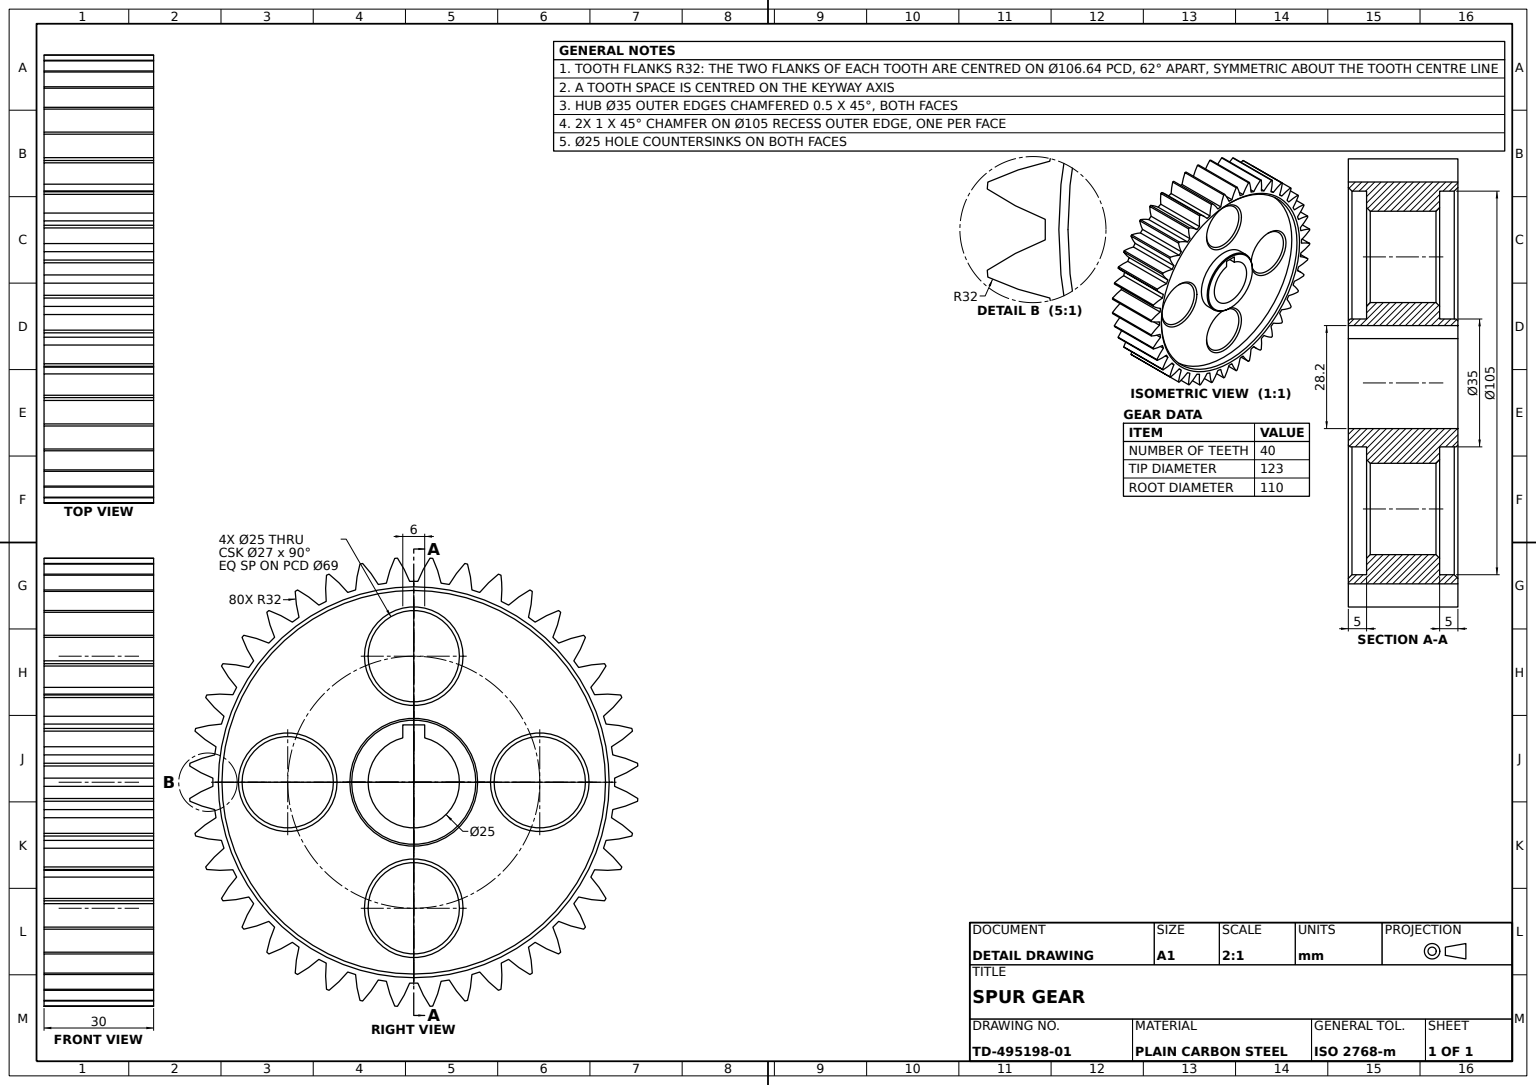
SolidWorks part; units mm, degrees
material "Plain Carbon Steel"
ref_plane "Front Plane" through (0, 0, 0) normal (0, 0, 1) x (1, 0, 0)
ref_plane "Top Plane" through (0, 0, 0) normal (0, 1, 0) x (1, 0, 0)
ref_plane "Right Plane" through (0, 0, 0) normal (1, 0, 0) x (0, 0, -1)
sketch "Gear Tooth Profile Sketch" plane through (0, 0, 0) normal (0, 0, 1) x (1, 0, 0)
  line L1 (3, 12.1347) -> (3, 15.7)
  line L2 (-3, 12.1347) -> (-3, 15.7)
  line L3 (-3, 15.7) -> (3, 15.7)
  arc A0 (-3, 12.1347) -> (3, 12.1347) centre (0, 0) ccw
  circle A1 centre (0, 0) radius 17.5
  circle A2 centre (0, 0) radius 52.5
  arc A3 (-13.9907, 59.8875) -> (-14.7225, 59.7118) centre (0, 0) ccw
  arc A4 (-15.9224, 52.6448) -> (-18.0623, 51.9495) centre (0, 0) ccw
  arc A5 (1.125, 54.9885) -> (4.45, 61.3388) centre (30.9582, 43.4135) cw
  arc A6 (-1.125, 54.9885) -> (-4.45, 61.3388) centre (-30.9582, 43.4135) ccw
  arc A7 (7.4909, 54.4875) -> (5.2003, 61.2797) centre (-23.7857, 47.722) ccw
  arc A8 (9.7132, 54.1355) -> (13.9907, 59.8875) centre (37.3684, 38.0361) cw
  arc A9 (15.9224, 52.6448) -> (14.7225, 59.7118) centre (-16.0275, 50.8553) ccw
  arc A10 (18.0623, 51.9495) -> (23.1869, 56.9615) centre (42.8585, 31.7221) cw
  arc A11 (23.9619, 49.5058) -> (23.8823, 56.6735) centre (-7.8746, 52.7365) ccw
  arc A12 (25.9666, 48.4844) -> (31.8122, 52.633) centre (47.2933, 24.627) cw
  arc A13 (31.4113, 45.1479) -> (32.4539, 52.2398) centre (0.4721, 53.3191) ccw
  arc A14 (33.2316, 43.8254) -> (39.6542, 47.0085) centre (50.5636, 16.9255) cw
  arc A15 (38.0872, 39.6782) -> (40.2265, 46.5197) centre (8.8072, 52.5888) ccw
  arc A16 (39.6782, 38.0872) -> (46.5197, 40.2265) centre (52.5888, 8.8072) cw
  arc A17 (43.8254, 33.2316) -> (47.0085, 39.6542) centre (16.9255, 50.5636) ccw
  arc A18 (45.1479, 31.4113) -> (52.2398, 32.4539) centre (53.3191, 0.4721) cw
  arc A19 (48.4844, 25.9666) -> (52.633, 31.8122) centre (24.627, 47.2933) ccw
  arc A20 (49.5058, 23.9619) -> (56.6735, 23.8823) centre (52.7365, -7.8746) cw
  arc A21 (51.9495, 18.0623) -> (56.9615, 23.1869) centre (31.7221, 42.8585) ccw
  arc A22 (52.6448, 15.9224) -> (59.7118, 14.7225) centre (50.8553, -16.0275) cw
  arc A23 (54.1355, 9.7132) -> (59.8875, 13.9907) centre (38.0361, 37.3684) ccw
  arc A24 (54.4875, 7.4909) -> (61.2797, 5.2003) centre (47.722, -23.7857) cw
  arc A25 (54.9885, 1.125) -> (61.3388, 4.45) centre (43.4135, 30.9582) ccw
  arc A26 (54.9885, -1.125) -> (61.3388, -4.45) centre (43.4135, -30.9582) cw
  arc A27 (54.4875, -7.4909) -> (61.2797, -5.2003) centre (47.722, 23.7857) ccw
  arc A28 (54.1355, -9.7132) -> (59.8875, -13.9907) centre (38.0361, -37.3684) cw
  arc A29 (52.6448, -15.9224) -> (59.7118, -14.7225) centre (50.8553, 16.0275) ccw
  arc A30 (51.9495, -18.0623) -> (56.9615, -23.1869) centre (31.7221, -42.8585) cw
  arc A31 (49.5058, -23.9619) -> (56.6735, -23.8823) centre (52.7365, 7.8746) ccw
  arc A32 (48.4844, -25.9666) -> (52.633, -31.8122) centre (24.627, -47.2933) cw
  arc A33 (45.1479, -31.4113) -> (52.2398, -32.4539) centre (53.3191, -0.4721) ccw
  arc A34 (43.8254, -33.2316) -> (47.0085, -39.6542) centre (16.9255, -50.5636) cw
  arc A35 (39.6782, -38.0872) -> (46.5197, -40.2265) centre (52.5888, -8.8072) ccw
  arc A36 (38.0872, -39.6782) -> (40.2265, -46.5197) centre (8.8072, -52.5888) cw
  arc A37 (33.2316, -43.8254) -> (39.6542, -47.0085) centre (50.5636, -16.9255) ccw
  arc A38 (31.4113, -45.1479) -> (32.4539, -52.2398) centre (0.4721, -53.3191) cw
  arc A39 (25.9666, -48.4844) -> (31.8122, -52.633) centre (47.2933, -24.627) ccw
  arc A40 (23.9619, -49.5058) -> (23.8823, -56.6735) centre (-7.8746, -52.7365) cw
  arc A41 (18.0623, -51.9495) -> (23.1869, -56.9615) centre (42.8585, -31.7221) ccw
  arc A42 (15.9224, -52.6448) -> (14.7225, -59.7118) centre (-16.0275, -50.8553) cw
  arc A43 (9.7132, -54.1355) -> (13.9907, -59.8875) centre (37.3684, -38.0361) ccw
  arc A44 (7.4909, -54.4875) -> (5.2003, -61.2797) centre (-23.7857, -47.722) cw
  arc A45 (1.125, -54.9885) -> (4.45, -61.3388) centre (30.9582, -43.4135) ccw
  arc A46 (-1.125, -54.9885) -> (-4.45, -61.3388) centre (-30.9582, -43.4135) cw
  arc A47 (-7.4909, -54.4875) -> (-5.2003, -61.2797) centre (23.7857, -47.722) ccw
  arc A48 (-9.7132, -54.1355) -> (-13.9907, -59.8875) centre (-37.3684, -38.0361) cw
  arc A49 (-15.9224, -52.6448) -> (-14.7225, -59.7118) centre (16.0275, -50.8553) ccw
  arc A50 (-18.0623, -51.9495) -> (-23.1869, -56.9615) centre (-42.8585, -31.7221) cw
  arc A51 (-23.9619, -49.5058) -> (-23.8823, -56.6735) centre (7.8746, -52.7365) ccw
  arc A52 (-25.9666, -48.4844) -> (-31.8122, -52.633) centre (-47.2933, -24.627) cw
  arc A53 (-31.4113, -45.1479) -> (-32.4539, -52.2398) centre (-0.4721, -53.3191) ccw
  arc A54 (-33.2316, -43.8254) -> (-39.6542, -47.0085) centre (-50.5636, -16.9255) cw
  arc A55 (-38.0872, -39.6782) -> (-40.2265, -46.5197) centre (-8.8072, -52.5888) ccw
  arc A56 (-39.6782, -38.0872) -> (-46.5197, -40.2265) centre (-52.5888, -8.8072) cw
  arc A57 (-43.8254, -33.2316) -> (-47.0085, -39.6542) centre (-16.9255, -50.5636) ccw
  arc A58 (-45.1479, -31.4113) -> (-52.2398, -32.4539) centre (-53.3191, -0.4721) cw
  arc A59 (-48.4844, -25.9666) -> (-52.633, -31.8122) centre (-24.627, -47.2933) ccw
  arc A60 (-49.5058, -23.9619) -> (-56.6735, -23.8823) centre (-52.7365, 7.8746) cw
  arc A61 (-51.9495, -18.0623) -> (-56.9615, -23.1869) centre (-31.7221, -42.8585) ccw
  arc A62 (-52.6448, -15.9224) -> (-59.7118, -14.7225) centre (-50.8553, 16.0275) cw
  arc A63 (-54.1355, -9.7132) -> (-59.8875, -13.9907) centre (-38.0361, -37.3684) ccw
  arc A64 (-54.4875, -7.4909) -> (-61.2797, -5.2003) centre (-47.722, 23.7857) cw
  arc A65 (-54.9885, -1.125) -> (-61.3388, -4.45) centre (-43.4135, -30.9582) ccw
  arc A66 (-54.9885, 1.125) -> (-61.3388, 4.45) centre (-43.4135, 30.9582) cw
  arc A67 (-54.4875, 7.4909) -> (-61.2797, 5.2003) centre (-47.722, -23.7857) ccw
  arc A68 (-54.1355, 9.7132) -> (-59.8875, 13.9907) centre (-38.0361, 37.3684) cw
  arc A69 (-52.6448, 15.9224) -> (-59.7118, 14.7225) centre (-50.8553, -16.0275) ccw
  arc A70 (-51.9495, 18.0623) -> (-56.9615, 23.1869) centre (-31.7221, 42.8585) cw
  arc A71 (-49.5058, 23.9619) -> (-56.6735, 23.8823) centre (-52.7365, -7.8746) ccw
  arc A72 (-48.4844, 25.9666) -> (-52.633, 31.8122) centre (-24.627, 47.2933) cw
  arc A73 (-45.1479, 31.4113) -> (-52.2398, 32.4539) centre (-53.3191, 0.4721) ccw
  arc A74 (-43.8254, 33.2316) -> (-47.0085, 39.6542) centre (-16.9255, 50.5636) cw
  arc A75 (-39.6782, 38.0872) -> (-46.5197, 40.2265) centre (-52.5888, 8.8072) ccw
  arc A76 (-38.0872, 39.6782) -> (-40.2265, 46.5197) centre (-8.8072, 52.5888) cw
  arc A77 (-33.2316, 43.8254) -> (-39.6542, 47.0085) centre (-50.5636, 16.9255) ccw
  arc A78 (-31.4113, 45.1479) -> (-32.4539, 52.2398) centre (-0.4721, 53.3191) cw
  arc A79 (-25.9666, 48.4844) -> (-31.8122, 52.633) centre (-47.2933, 24.627) ccw
  arc A80 (-23.9619, 49.5058) -> (-23.8823, 56.6735) centre (7.8746, 52.7365) cw
  arc A81 (-18.0623, 51.9495) -> (-23.1869, 56.9615) centre (-42.8585, 31.7221) ccw
  arc A82 (-15.9224, 52.6448) -> (-14.7225, 59.7118) centre (16.0275, 50.8553) cw
  arc A83 (-9.7132, 54.1355) -> (-13.9907, 59.8875) centre (-37.3684, 38.0361) ccw
  arc A84 (-7.4909, 54.4875) -> (-5.2003, 61.2797) centre (23.7857, 47.722) cw
  arc A85 (-23.1869, 56.9615) -> (-23.8823, 56.6735) centre (0, 0) ccw
  arc A86 (-31.8122, 52.633) -> (-32.4539, 52.2398) centre (0, 0) ccw
  arc A87 (-39.6542, 47.0085) -> (-40.2265, 46.5197) centre (0, 0) ccw
  arc A88 (-46.5197, 40.2265) -> (-47.0085, 39.6542) centre (0, 0) ccw
  arc A89 (-52.2398, 32.4539) -> (-52.633, 31.8122) centre (0, 0) ccw
  arc A90 (-4.45, 61.3388) -> (-5.2003, 61.2797) centre (0, 0) ccw
  arc A91 (5.2003, 61.2797) -> (4.45, 61.3388) centre (0, 0) ccw
  arc A92 (14.7225, 59.7118) -> (13.9907, 59.8875) centre (0, 0) ccw
  arc A93 (23.8823, 56.6735) -> (23.1869, 56.9615) centre (0, 0) ccw
  arc A94 (32.4539, 52.2398) -> (31.8122, 52.633) centre (0, 0) ccw
  arc A95 (40.2265, 46.5197) -> (39.6542, 47.0085) centre (0, 0) ccw
  arc A96 (47.0085, 39.6542) -> (46.5197, 40.2265) centre (0, 0) ccw
  arc A97 (-56.6735, 23.8823) -> (-56.9615, 23.1869) centre (0, 0) ccw
  arc A98 (-59.7118, 14.7225) -> (-59.8875, 13.9907) centre (0, 0) ccw
  arc A99 (-61.2797, 5.2003) -> (-61.3388, 4.45) centre (0, 0) ccw
  arc A100 (-61.3388, -4.45) -> (-61.2797, -5.2003) centre (0, 0) ccw
  arc A101 (-59.8875, -13.9907) -> (-59.7118, -14.7225) centre (0, 0) ccw
  arc A102 (-56.9615, -23.1869) -> (-56.6735, -23.8823) centre (0, 0) ccw
  arc A103 (-52.633, -31.8122) -> (-52.2398, -32.4539) centre (0, 0) ccw
  arc A104 (-47.0085, -39.6542) -> (-46.5197, -40.2265) centre (0, 0) ccw
  arc A105 (-40.2265, -46.5197) -> (-39.6542, -47.0085) centre (0, 0) ccw
  arc A106 (-32.4539, -52.2398) -> (-31.8122, -52.633) centre (0, 0) ccw
  arc A107 (-23.8823, -56.6735) -> (-23.1869, -56.9615) centre (0, 0) ccw
  arc A108 (-14.7225, -59.7118) -> (-13.9907, -59.8875) centre (0, 0) ccw
  arc A109 (-5.2003, -61.2797) -> (-4.45, -61.3388) centre (0, 0) ccw
  arc A110 (4.45, -61.3388) -> (5.2003, -61.2797) centre (0, 0) ccw
  arc A111 (13.9907, -59.8875) -> (14.7225, -59.7118) centre (0, 0) ccw
  arc A112 (23.1869, -56.9615) -> (23.8823, -56.6735) centre (0, 0) ccw
  arc A113 (31.8122, -52.633) -> (32.4539, -52.2398) centre (0, 0) ccw
  arc A114 (39.6542, -47.0085) -> (40.2265, -46.5197) centre (0, 0) ccw
  arc A115 (46.5197, -40.2265) -> (47.0085, -39.6542) centre (0, 0) ccw
  arc A116 (52.2398, -32.4539) -> (52.633, -31.8122) centre (0, 0) ccw
  arc A117 (56.6735, -23.8823) -> (56.9615, -23.1869) centre (0, 0) ccw
  arc A118 (59.7118, -14.7225) -> (59.8875, -13.9907) centre (0, 0) ccw
  arc A119 (61.2797, -5.2003) -> (61.3388, -4.45) centre (0, 0) ccw
  arc A120 (61.3388, 4.45) -> (61.2797, 5.2003) centre (0, 0) ccw
  arc A121 (59.8875, 13.9907) -> (59.7118, 14.7225) centre (0, 0) ccw
  arc A122 (56.9615, 23.1869) -> (56.6735, 23.8823) centre (0, 0) ccw
  arc A123 (52.633, 31.8122) -> (52.2398, 32.4539) centre (0, 0) ccw
  arc A124 (-7.4909, 54.4875) -> (-9.7132, 54.1355) centre (0, 0) ccw
  arc A125 (1.125, 54.9885) -> (-1.125, 54.9885) centre (0, 0) ccw
  arc A126 (9.7132, 54.1355) -> (7.4909, 54.4875) centre (0, 0) ccw
  arc A127 (18.0623, 51.9495) -> (15.9224, 52.6448) centre (0, 0) ccw
  arc A128 (25.9666, 48.4844) -> (23.9619, 49.5058) centre (0, 0) ccw
  arc A129 (33.2316, 43.8254) -> (31.4113, 45.1479) centre (0, 0) ccw
  arc A130 (39.6782, 38.0872) -> (38.0872, 39.6782) centre (0, 0) ccw
  arc A131 (45.1479, 31.4113) -> (43.8254, 33.2316) centre (0, 0) ccw
  arc A132 (49.5058, 23.9619) -> (48.4844, 25.9666) centre (0, 0) ccw
  arc A133 (52.6448, 15.9224) -> (51.9495, 18.0623) centre (0, 0) ccw
  arc A134 (54.4875, 7.4909) -> (54.1355, 9.7132) centre (0, 0) ccw
  arc A135 (54.9885, -1.125) -> (54.9885, 1.125) centre (0, 0) ccw
  arc A136 (54.1355, -9.7132) -> (54.4875, -7.4909) centre (0, 0) ccw
  arc A137 (51.9495, -18.0623) -> (52.6448, -15.9224) centre (0, 0) ccw
  arc A138 (48.4844, -25.9666) -> (49.5058, -23.9619) centre (0, 0) ccw
  arc A139 (43.8254, -33.2316) -> (45.1479, -31.4113) centre (0, 0) ccw
  arc A140 (38.0872, -39.6782) -> (39.6782, -38.0872) centre (0, 0) ccw
  arc A141 (31.4113, -45.1479) -> (33.2316, -43.8254) centre (0, 0) ccw
  arc A142 (23.9619, -49.5058) -> (25.9666, -48.4844) centre (0, 0) ccw
  arc A143 (15.9224, -52.6448) -> (18.0623, -51.9495) centre (0, 0) ccw
  arc A144 (7.4909, -54.4875) -> (9.7132, -54.1355) centre (0, 0) ccw
  arc A145 (-1.125, -54.9885) -> (1.125, -54.9885) centre (0, 0) ccw
  arc A146 (-9.7132, -54.1355) -> (-7.4909, -54.4875) centre (0, 0) ccw
  arc A147 (-18.0623, -51.9495) -> (-15.9224, -52.6448) centre (0, 0) ccw
  arc A148 (-25.9666, -48.4844) -> (-23.9619, -49.5058) centre (0, 0) ccw
  arc A149 (-23.9619, 49.5058) -> (-25.9666, 48.4844) centre (0, 0) ccw
  arc A150 (-31.4113, 45.1479) -> (-33.2316, 43.8254) centre (0, 0) ccw
  arc A151 (-38.0872, 39.6782) -> (-39.6782, 38.0872) centre (0, 0) ccw
  arc A152 (-43.8254, 33.2316) -> (-45.1479, 31.4113) centre (0, 0) ccw
  arc A153 (-48.4844, 25.9666) -> (-49.5058, 23.9619) centre (0, 0) ccw
  arc A154 (-51.9495, 18.0623) -> (-52.6448, 15.9224) centre (0, 0) ccw
  arc A155 (-54.1355, 9.7132) -> (-54.4875, 7.4909) centre (0, 0) ccw
  arc A156 (-54.9885, 1.125) -> (-54.9885, -1.125) centre (0, 0) ccw
  arc A157 (-54.4875, -7.4909) -> (-54.1355, -9.7132) centre (0, 0) ccw
  arc A158 (-52.6448, -15.9224) -> (-51.9495, -18.0623) centre (0, 0) ccw
  arc A159 (-49.5058, -23.9619) -> (-48.4844, -25.9666) centre (0, 0) ccw
  arc A160 (-45.1479, -31.4113) -> (-43.8254, -33.2316) centre (0, 0) ccw
  arc A161 (-39.6782, -38.0872) -> (-38.0872, -39.6782) centre (0, 0) ccw
  arc A162 (-33.2316, -43.8254) -> (-31.4113, -45.1479) centre (0, 0) ccw
  point P4 (3, 0)
  point P5 (3, 15.7)
  point P7 (-3, 0)
  dimension "D1" = 25
  dimension "D2" = 35
  dimension "D8" = 105
  dimension "D9" = 123
  dimension "D10" = 110
  dimension "D13" = 32
  dimension "D19" = 32
  dimension "D21" = 40
  dimension "D3" = 15.7
  dimension "D5" = 3
  dimension "D4" = 3
  dimension "D6" = 12.1347
  dimension "D7" = 12.1347
  dimension "D11" = 1.125
  dimension "D12" = 2.25
  dimension "D15" = 4.45
  dimension "D20" = 8.9
extrude "Gear Blank 30mm" add sketch "Gear Tooth Profile Sketch" along normal blind 30 contours A2 A1 | A54 A162 A53 A106 A52 A148 A51 A107 A50 A147 A49 A108 A48 A146 A47 A109 A46 A145 A45 A110 A44 A144 A43 A111 A42 A143 A41 A112 A40 A142 A39 A113 A38 A141 A37 A114 A36 A140 A35 A115 A34 A139 A33 A116 A32 A138 A31 A117 A30 A137 A29
sketch "Front Recess Sketch Ø105" plane through (0, 0, 30) normal (0, 0, 1) x (1, 0, 0)
  circle A0 centre (0, 0) radius 52.5
  dimension "D1" = 105
extrude "Front Web Recess Ø105x5" cut sketch "Front Recess Sketch Ø105" against normal blind 5
sketch "Rear Recess Sketch Ø105" plane through (0, 0, 0) normal (0, 0, -1) x (-1, 0, 0)
  circle A0 centre (0, 0) radius 52.5
  dimension "D1" = 105
extrude "Rear Web Recess Ø105x5" cut sketch "Rear Recess Sketch Ø105" against normal blind 5
chamfer "Rear Recess Chamfer 1mm" distance 1 angle 45 1 edges at (-52.5, 0, 0)
chamfer "Front Recess Chamfer 1mm" distance 1 angle 45 1 edges at (52.5, 0, 30)
sketch "Hub Sketch Ø35" plane through (0, 0, 25) normal (0, 0, 1) x (1, 0, 0)
  circle A0 centre (0, 0) radius 17.5
  dimension "D1" = 35
extrude "Hub Ø35" add sketch "Hub Sketch Ø35" against normal blind 20
sketch "Keyed Bore Sketch" plane through (0, 0, 25) normal (0, 0, 1) x (1, 0, 0)
  line L1 (3, 12.1347) -> (3, 15.7)
  line L2 (-3, 12.1347) -> (-3, 15.7)
  line L3 (-3, 15.7) -> (3, 15.7)
  arc A1 (-3, 12.1347) -> (3, 12.1347) centre (0, 0) ccw
  point P4 (3, 0)
  point P5 (0, 15.7)
  point P7 (-3, 0)
  dimension "D2" = 25
  dimension "D3" = 6
  dimension "D5" = 12.1347
  dimension "D4" = 3
  dimension "D6" = 15.7
  dimension "D7" = 12.1347
extrude "Keyed Bore Ø25" cut sketch "Keyed Bore Sketch" against normal blind 20
sketch "Front Hub Boss Sketch" plane through (0, 0, 25) normal (0, 0, 1) x (1, 0, 0)
  line L0 (-3, 12.1347) -> (-3, 15.7)
  line L1 (-3, 15.7) -> (3, 15.7)
  line L2 (3, 15.7) -> (3, 12.1347)
  circle A0 centre (0, 0) radius 17.5
  arc A1 (-3, 12.1347) -> (3, 12.1347) centre (0, 0) ccw
  dimension "D1" = 35
extrude "Front Hub Boss Ø35x5" add sketch "Front Hub Boss Sketch" along normal blind 5
sketch "Rear Hub Boss Sketch" plane through (0, 0, 5) normal (0, 0, -1) x (-1, 0, 0)
  line L0 (-3, 12.1347) -> (-3, 15.7)
  line L1 (-3, 15.7) -> (3, 15.7)
  line L2 (3, 15.7) -> (3, 12.1347)
  arc A0 (-3, 12.1347) -> (3, 12.1347) centre (0, 0) ccw
  circle A1 centre (0, 0) radius 17.5
  dimension "D1" = 35
extrude "Rear Hub Boss Ø35x5" add sketch "Rear Hub Boss Sketch" along normal blind 5
sketch "Lightening Holes Sketch 4xØ25" plane through (0, 0, 25) normal (0, 0, 1) x (1, 0, 0)
  circle A0 centre (0, 34.5) radius 12.5
  circle A2 centre (34.5, 0) radius 12.5
  circle A3 centre (0, -34.5) radius 12.5
  circle A4 centre (-34.5, 0) radius 12.5
  dimension "D1" = 25
  dimension "D2" = 34.5
  dimension "D3" = 61.3388
  dimension "D5" = 34.5
  dimension "D6" = 61.3388
  dimension "D4" = 4
extrude "Lightening Holes 4xØ25" cut sketch "Lightening Holes Sketch 4xØ25" against normal blind 20
chamfer "Lightening Hole Chamfers 1mm" distance 1 angle 45 8 edges at (12.5, -34.5, 5) (12.5, -34.5, 25) (47, 0, 5) (47, 0, 25) (-22, 0, 5) (-22, 0, 25) (12.5, 34.5, 5) (12.5, 34.5, 25)
chamfer "Front Hub Chamfer 0.5mm" distance 0.5 angle 45 1 edges at (17.5, 0, 30)
chamfer "Rear Hub Chamfer 0.5mm" distance 0.5 angle 45 1 edges at (-17.5, 0, 0)
